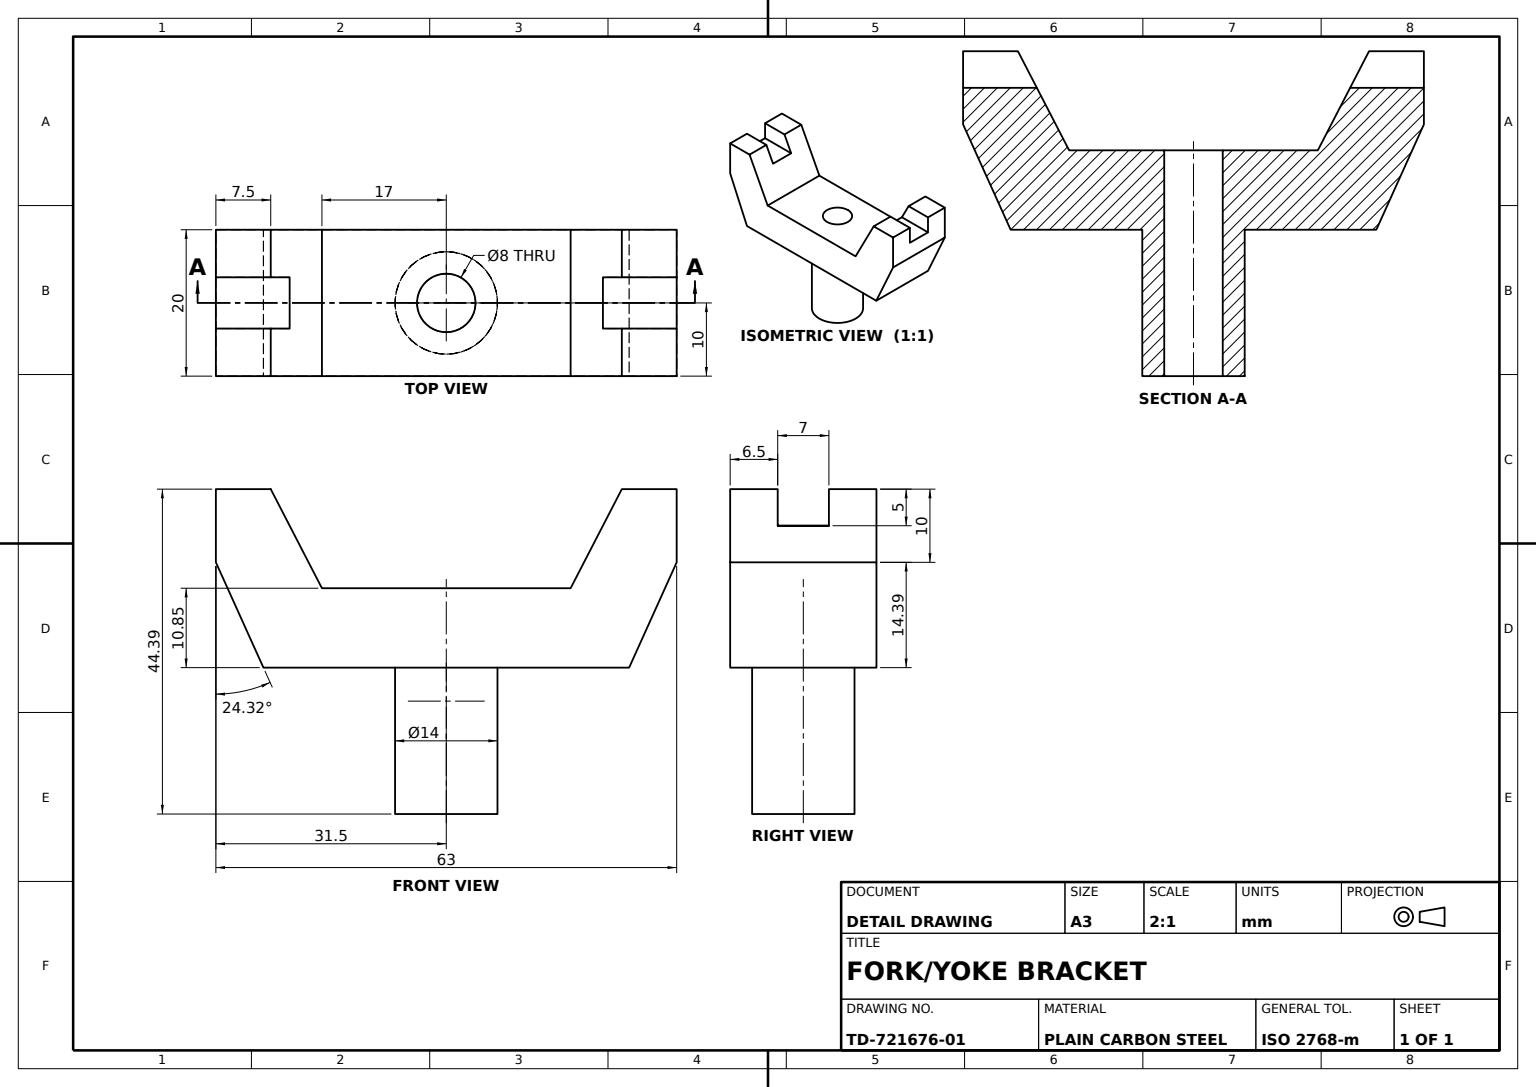
from build123d import *

# Parameters (mm, degrees)
YOKE_BODY_DEPTH      = 10
ARM_SLOTS_DEPTH      = 66.209374322
POST_SEAT_SKETCH_R   = 4
POST_SEAT_CUT_DEPTH  = 20
PIVOT_POST_SKETCH_R  = 7
PIVOT_POST_DEPTH     = 20
CENTRE_HOLE_SKETCH_R = 4
CENTRE_HOLE_DEPTH    = 46.209194984


with BuildPart() as part:
    # Yoke Profile Sketch → Yoke Body (new, symmetric)
    with BuildSketch(Plane.XY):
        Polygon((0, 0), (17, 0), (24, 13.537448042), (31.5, 13.537448042), (31.5, 3.537448042), (25, -10.848359941), (-25, -10.848359941), (-31.5, 3.537448042), (-31.5, 13.537448042), (-24, 13.537448042), (-17, 0), align=None)
    extrude(amount=YOKE_BODY_DEPTH, both=True)

    # Arm Slots Sketch → Arm Slots (cut, through all)
    with BuildSketch(Plane.ZY.offset(31.5)):
        Polygon((0, 13.537448042), (3.5, 13.537448042), (3.5, 8.537448042), (-3.5, 8.537448042), (-3.5, 13.537448042), align=None)
    extrude(amount=-ARM_SLOTS_DEPTH, mode=Mode.SUBTRACT)

    # Post Seat Sketch → Post Seat Cut (cut)
    with BuildSketch(Plane(origin=(0, 0, 0), x_dir=(1, 0, 0), z_dir=(0, 1, 0))):
        with Locations(Location((0, 0, 0), (0, 0, 270))):
            Circle(POST_SEAT_SKETCH_R)
    extrude(amount=-POST_SEAT_CUT_DEPTH, mode=Mode.SUBTRACT)

    # Pivot Post Sketch → Pivot Post (add)
    with BuildSketch(Plane.XZ.offset(10.848359941)):
        with Locations(Location((0, 0, 0), (0, 0, 90))):
            Circle(PIVOT_POST_SKETCH_R)
    extrude(amount=PIVOT_POST_DEPTH)

    # Centre Hole Sketch → Centre Hole (cut, through all)
    with BuildSketch(Plane(origin=(0, 0, 0), x_dir=(1, 0, 0), z_dir=(0, 1, 0))):
        with Locations(Location((0, 0, 0), (0, 0, 270))):
            Circle(CENTRE_HOLE_SKETCH_R)
    extrude(amount=-CENTRE_HOLE_DEPTH, mode=Mode.SUBTRACT)


solid = part.part
